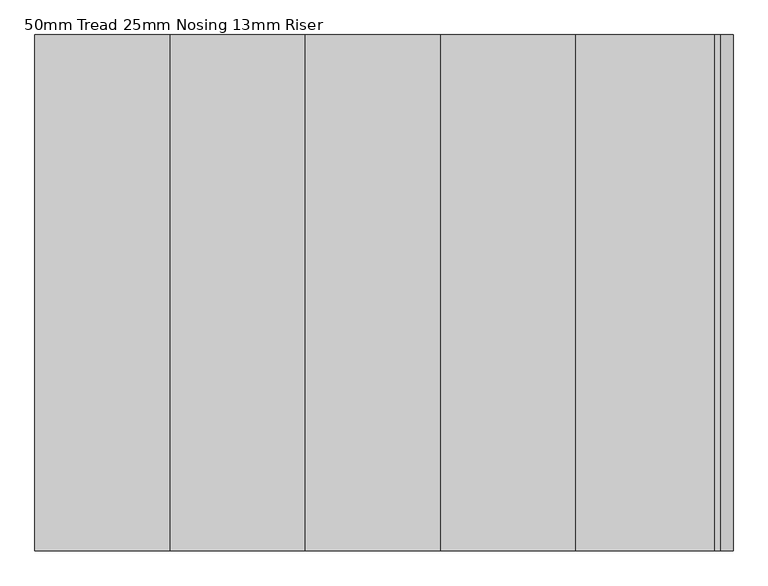
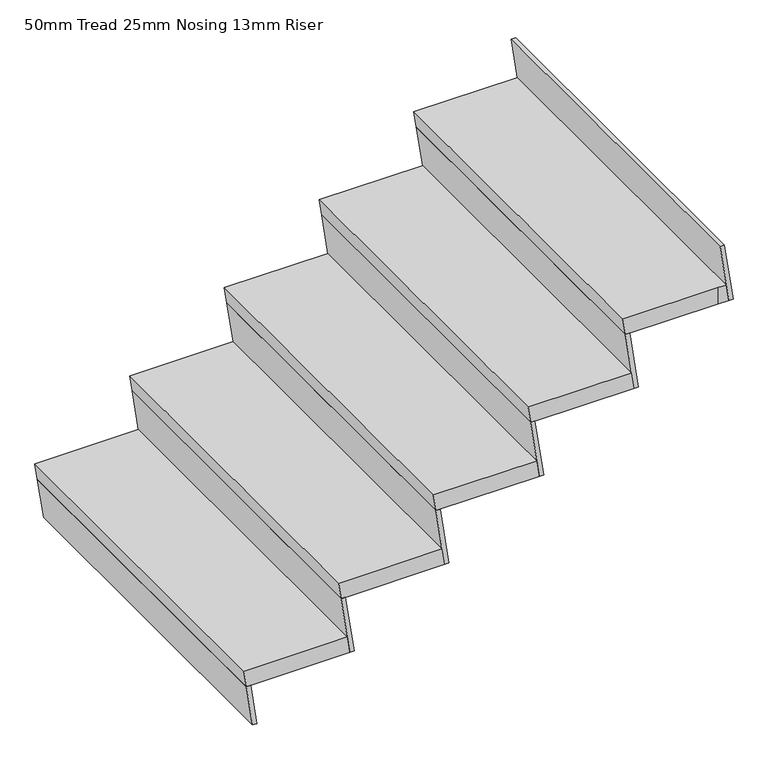
"""IFC4 building model written with IfcOpenShell, lengths in millimetres: stair flight geometry, 50mm Tread 25mm Nosing 13mm Riser."""

from ifc_helpers import new_model, si_unit, origin, place, context, project, spatial, faceted_brep, source, transform, mapped, element, save


def stair_flight_50mm_tread_25mm_nosing_13mm_riser_430ad9a4(model_context):
    return source(origin(), model_context, "Body", "Brep", [
        faceted_brep([(-228.272677, 3071.4281795, 347.826087), (-221.085177, 3071.4281795, 297.826087), (-221.085177, 4121.4539608, 297.826087), (-228.272677, 4121.4539608, 347.826087), (-528.272677, 4121.4539608, 347.826087), (-528.272677, 3071.4281795, 347.826087), (-521.085177, 3071.4281795, 297.826087), (-521.085177, 4121.4539608, 297.826087)], [[[0, 1, 2, 3]], [[3, 4, 5, 0]], [[2, 1, 6, 7]], [[4, 3, 2, 7]], [[0, 5, 6, 1]], [[5, 4, 7, 6]]]),
        faceted_brep([(-521.085177, 3071.4281795, 297.826087), (-503.272677, 3071.4281795, 173.9130435), (-490.644187, 3071.4281795, 173.9130435), (-508.456687, 3071.4281795, 297.826087), (-521.085177, 4121.4539608, 297.826087), (-508.456687, 4121.4539608, 297.826087), (-490.644187, 4121.4539608, 173.9130435), (-503.272677, 4121.4539608, 173.9130435)], [[[0, 1, 2, 3]], [[4, 5, 6, 7]], [[1, 0, 4, 7]], [[2, 1, 7, 6]], [[3, 2, 6, 5]], [[0, 3, 5, 4]]]),
        faceted_brep([(-246.085177, 3071.4281795, 471.7391304), (-221.085177, 3071.4281795, 297.826087), (-208.456687, 3071.4281795, 297.826087), (-233.456687, 3071.4281795, 471.7391304), (-246.085177, 4121.4539608, 471.7391304), (-233.456687, 4121.4539608, 471.7391304), (-208.456687, 4121.4539608, 297.826087), (-221.085177, 4121.4539608, 297.826087)], [[[0, 1, 2, 3]], [[4, 5, 6, 7]], [[1, 0, 4, 7]], [[2, 1, 7, 6]], [[3, 2, 6, 5]], [[0, 3, 5, 4]]]),
        faceted_brep([(46.727323, 4121.4539608, 521.7391304), (-253.272677, 4121.4539608, 521.7391304), (-253.272677, 3071.4281795, 521.7391304), (46.727323, 3071.4281795, 521.7391304), (53.914823, 4121.4539608, 471.7391304), (53.914823, 3071.4281795, 471.7391304), (-246.085177, 3071.4281795, 471.7391304), (-246.085177, 4121.4539608, 471.7391304)], [[[0, 1, 2, 3]], [[4, 5, 6, 7]], [[1, 0, 4, 7]], [[3, 2, 6, 5]], [[3, 5, 4, 0]], [[2, 1, 7, 6]]]),
        faceted_brep([(28.914823, 3071.4281795, 645.6521739), (53.914823, 3071.4281795, 471.7391304), (66.543313, 3071.4281795, 471.7391304), (41.543313, 3071.4281795, 645.6521739), (28.914823, 4121.4539608, 645.6521739), (41.543313, 4121.4539608, 645.6521739), (66.543313, 4121.4539608, 471.7391304), (53.914823, 4121.4539608, 471.7391304)], [[[0, 1, 2, 3]], [[4, 5, 6, 7]], [[1, 0, 4, 7]], [[2, 1, 7, 6]], [[3, 2, 6, 5]], [[0, 3, 5, 4]]]),
        faceted_brep([(321.727323, 4121.4539608, 695.6521739), (21.727323, 4121.4539608, 695.6521739), (21.727323, 3071.4281795, 695.6521739), (321.727323, 3071.4281795, 695.6521739), (328.914823, 4121.4539608, 645.6521739), (328.914823, 3071.4281795, 645.6521739), (28.914823, 3071.4281795, 645.6521739), (28.914823, 4121.4539608, 645.6521739)], [[[0, 1, 2, 3]], [[4, 5, 6, 7]], [[1, 0, 4, 7]], [[3, 2, 6, 5]], [[3, 5, 4, 0]], [[2, 1, 7, 6]]]),
        faceted_brep([(303.914823, 3071.4281795, 819.5652174), (328.914823, 3071.4281795, 645.6521739), (341.543313, 3071.4281795, 645.6521739), (316.543313, 3071.4281795, 819.5652174), (303.914823, 4121.4539608, 819.5652174), (316.543313, 4121.4539608, 819.5652174), (341.543313, 4121.4539608, 645.6521739), (328.914823, 4121.4539608, 645.6521739)], [[[0, 1, 2, 3]], [[4, 5, 6, 7]], [[1, 0, 4, 7]], [[2, 1, 7, 6]], [[3, 2, 6, 5]], [[0, 3, 5, 4]]]),
        faceted_brep([(596.727323, 4121.4539608, 869.5652174), (296.727323, 4121.4539608, 869.5652174), (296.727323, 3071.4281795, 869.5652174), (596.727323, 3071.4281795, 869.5652174), (603.914823, 4121.4539608, 819.5652174), (603.914823, 3071.4281795, 819.5652174), (303.914823, 3071.4281795, 819.5652174), (303.914823, 4121.4539608, 819.5652174)], [[[0, 1, 2, 3]], [[4, 5, 6, 7]], [[1, 0, 4, 7]], [[3, 2, 6, 5]], [[3, 5, 4, 0]], [[2, 1, 7, 6]]]),
        faceted_brep([(578.914823, 3071.4281795, 993.4782609), (603.914823, 3071.4281795, 819.5652174), (616.543313, 3071.4281795, 819.5652174), (591.543313, 3071.4281795, 993.4782609), (578.914823, 4121.4539608, 993.4782609), (591.543313, 4121.4539608, 993.4782609), (616.543313, 4121.4539608, 819.5652174), (603.914823, 4121.4539608, 819.5652174)], [[[0, 1, 2, 3]], [[4, 5, 6, 7]], [[1, 0, 4, 7]], [[2, 1, 7, 6]], [[3, 2, 6, 5]], [[0, 3, 5, 4]]]),
        faceted_brep([(853.914823, 3071.4281795, 1167.3913043), (878.914823, 3071.4281795, 993.4782609), (891.543313, 3071.4281795, 993.4782609), (866.543313, 3071.4281795, 1167.3913043), (853.914823, 4121.4539608, 1167.3913043), (866.543313, 4121.4539608, 1167.3913043), (891.543313, 4121.4539608, 993.4782609), (878.914823, 4121.4539608, 993.4782609)], [[[0, 1, 2, 3]], [[4, 5, 6, 7]], [[1, 0, 4, 7]], [[2, 1, 7, 6]], [[3, 2, 6, 5]], [[0, 3, 5, 4]]]),
        faceted_brep([(871.727323, 4121.4539608, 1043.4782609), (571.727323, 4121.4539608, 1043.4782609), (571.727323, 3071.4281795, 1043.4782609), (846.727323, 3071.4281795, 1043.4782609), (871.727323, 3071.4281795, 1043.4782609), (878.914823, 4121.4539608, 993.4782609), (878.914823, 3071.4281795, 993.4782609), (846.727323, 3071.4281795, 993.4782609), (578.914823, 3071.4281795, 993.4782609), (578.914823, 4121.4539608, 993.4782609)], [[[0, 1, 2, 3, 4]], [[5, 6, 7, 8, 9]], [[1, 0, 5, 9]], [[3, 2, 8, 7]], [[4, 3, 7, 6]], [[4, 6, 5, 0]], [[2, 1, 9, 8]]]),
    ])


if __name__ == "__main__":
    model = new_model("IFC4")
    model_context = context("Model", 3, world=origin())
    ifc_project = project(units=[si_unit("LENGTHUNIT", "METRE", prefix="MILLI")], contexts=[model_context])
    site = spatial("IfcSite", under=ifc_project)
    building = spatial("IfcBuilding", under=site)
    placement = place(None, origin())
    stair_flight_50mm_tread_25mm_nosing_13mm_riser_shape = stair_flight_50mm_tread_25mm_nosing_13mm_riser_430ad9a4(model_context)
    element("IfcStairFlight", 1, ObjectType="50mm Tread 25mm Nosing 13mm Riser", at=placement, inside=building, context=model_context, shape_type="MappedRepresentation", body=[
        mapped(stair_flight_50mm_tread_25mm_nosing_13mm_riser_shape, transform((0.0, 0.0, 0.0), x_axis=(1.0, 0.0, 0.0), y_axis=(0.0, 1.0, 0.0), z_axis=(0.0, 0.0, 1.0))),
    ])
    save(model, "model.ifc")
